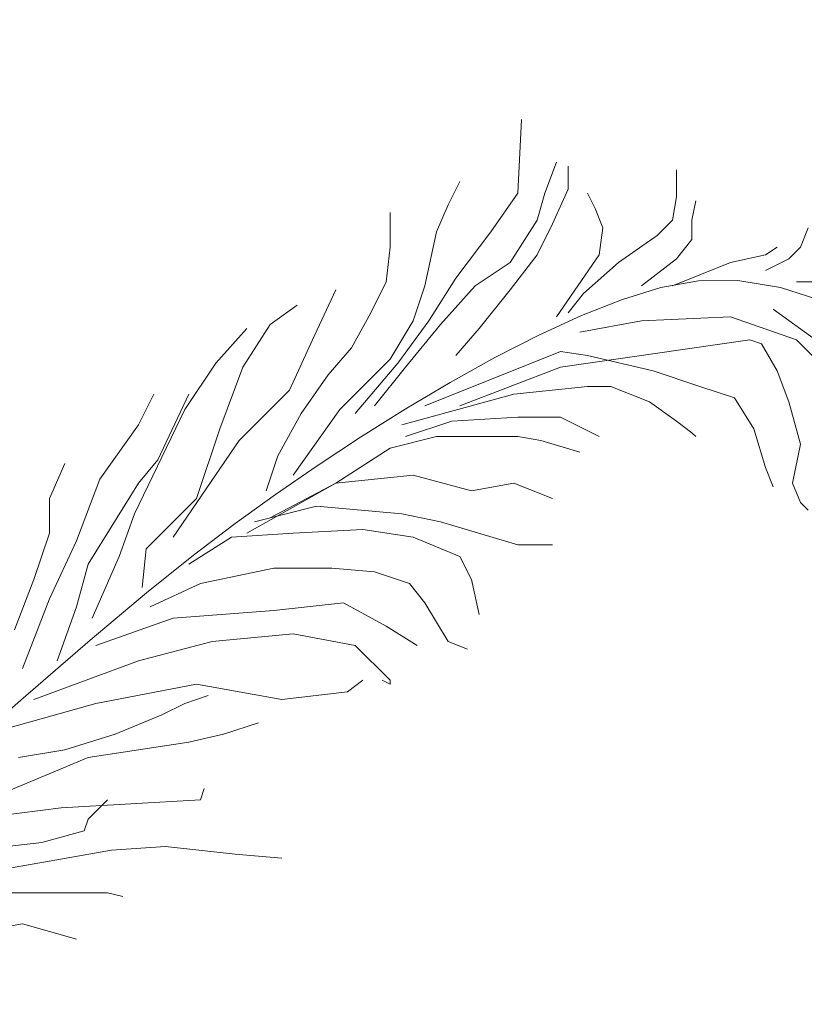
# Model space of a CAD drawing. Units: millimetres. Extents: x 595116 to 630915, y 909473 to 920225.
# Tile 62 of 134: x 629604.389 to 629608.928, y 919295.882 to 919301.582. Entities that reach past the tile are written whole.
import ezdxf

# ---------------------------------------------------------------- set-up
doc = ezdxf.new("R2010")
doc.units = ezdxf.units.MM
doc.layers.add('Dimension', color=3, linetype='Continuous', lineweight=18)
doc.layers.add('L-PLNT', color=85, linetype='Continuous', lineweight=13)
doc.styles.get("Standard").update_dxf_attribs({"font": 'arial.ttf'})
doc.dimstyles.new('ISO-25', dxfattribs={"dimtxt": 9, "dimasz": 6, "dimexe": 1.25, "dimexo": 0.625, "dimtad": 1, "dimlunit": 4, "dimtxsty": 'Standard', "dimcen": 2.5, "dimadec": 0, "dimazin": 0, "dimtfac": 1, "dimtmove": 0, "dimatfit": 3, "dimfxl": 1, "dimarcsym": 0})

# ---------------------------------------------------------------- blocks, each defined once
blk = doc.blocks.new('A$C4FB75ABC')
for p, q in [((4.1608, 3.5609), (4.1668, 3.6742)), ((4.2026, 3.5609), (4.2205, 3.6086)), ((4.2384, 3.5668), (4.2384, 3.6026)), ((4.4054, 3.5549), (4.4054, 3.5967)), ((4.0535, 3.543), (4.0714, 3.5788)), ((4.1191, 3.5013), (4.1608, 3.5609)), ((4.1907, 3.5192), (4.2026, 3.5609)), ((4.2145, 3.5132), (4.2384, 3.5668)), ((4.2801, 3.537), (4.2682, 3.5609)), ((4.3994, 3.5192), (4.4054, 3.5549)), ((4.0356, 3.5013), (4.0535, 3.543)), ((4.4293, 3.5192), (4.4352, 3.549)), ((3.964, 3.4774), (3.964, 3.5311)), ((4.2921, 3.5072), (4.2801, 3.537)), ((4.1489, 3.4536), (4.1907, 3.5192)), ((4.1907, 3.4655), (4.2145, 3.5132)), ((4.3756, 3.4953), (4.3994, 3.5192)), ((4.4293, 3.4893), (4.4293, 3.5192)), ((4.0177, 3.4178), (4.0356, 3.5013)), ((4.0654, 3.4297), (4.1191, 3.5013)), ((4.2861, 3.4655), (4.2921, 3.5072)), ((4.3159, 3.4536), (4.3756, 3.4953)), ((4.5963, 3.4774), (4.6082, 3.5072)), ((3.958, 3.4238), (3.964, 3.4774)), ((4.4054, 3.4595), (4.4293, 3.4893)), ((4.5426, 3.4655), (4.5605, 3.4774)), ((4.5784, 3.4595), (4.5963, 3.4774)), ((4.1489, 3.4118), (4.1907, 3.4655)), ((4.2205, 3.3701), (4.2861, 3.4655)), ((4.4889, 3.4536), (4.5426, 3.4655)), ((4.0952, 3.4178), (4.1489, 3.4536)), ((4.2622, 3.4059), (4.3159, 3.4536)), ((4.3517, 3.4178), (4.4054, 3.4595)), ((4.3994, 3.4178), (4.4889, 3.4536)), ((4.5426, 3.4416), (4.5784, 3.4595)), ((3.9342, 3.3761), (3.958, 3.4238)), ((3.9998, 3.3641), (4.0177, 3.4178)), ((4.0237, 3.3641), (4.0654, 3.4297)), ((4.0415, 3.3582), (4.0952, 3.4178)), ((4.3813, 3.4152), (4.4396, 3.4254)), ((4.4396, 3.4254), (4.5001, 3.426)), ((4.5001, 3.426), (4.5657, 3.4153)), ((4.5903, 3.4238), (4.6201, 3.4238)), ((3.8447, 3.3343), (3.8805, 3.4118)), ((4.1012, 3.3522), (4.1489, 3.4118)), ((4.2384, 3.3761), (4.2622, 3.4059)), ((4.322, 3.3969), (4.3813, 3.4152)), ((4.5657, 3.4153), (4.6395, 3.3917)), ((3.7791, 3.3582), (3.8208, 3.388)), ((4.2593, 3.3722), (4.322, 3.3969)), ((3.9044, 3.3224), (3.9342, 3.3761)), ((4.1935, 3.342), (4.2593, 3.3722)), ((4.5545, 3.382), (4.6858, 3.2866)), ((3.7373, 3.2926), (3.7791, 3.3582)), ((3.964, 3.3045), (3.9998, 3.3641)), ((3.9759, 3.2986), (4.0237, 3.3641)), ((3.9879, 3.2926), (4.0415, 3.3582)), ((4.2563, 3.3463), (4.3517, 3.3641)), ((4.3517, 3.3641), (4.4889, 3.3701)), ((4.4889, 3.3701), (4.5903, 3.3343)), ((3.6956, 3.2986), (3.7433, 3.3522)), ((4.0654, 3.3105), (4.1012, 3.3522)), ((4.1256, 3.3072), (4.1935, 3.342)), ((3.8089, 3.2568), (3.8447, 3.3343)), ((4.2265, 3.2926), (4.5187, 3.3343)), ((4.5187, 3.3343), (4.5366, 3.3284)), ((4.5366, 3.3284), (4.5605, 3.2866)), ((4.5903, 3.3343), (4.644, 3.2807)), ((3.8686, 3.2807), (3.9044, 3.3224)), ((4.0177, 3.233), (4.2265, 3.3164)), ((4.2265, 3.3164), (4.2682, 3.3105)), ((4.2682, 3.3105), (4.3696, 3.2866)), ((3.6479, 3.227), (3.6956, 3.2986)), ((3.8865, 3.227), (3.964, 3.3045)), ((3.9103, 3.2211), (3.9759, 3.2986)), ((4.0565, 3.2687), (4.1256, 3.3072)), ((3.7015, 3.1972), (3.7373, 3.2926)), ((3.8268, 3.2211), (3.8686, 3.2807)), ((3.9401, 3.233), (3.9879, 3.2926)), ((4.0714, 3.233), (4.2265, 3.2926)), ((4.3696, 3.2866), (4.4412, 3.2628)), ((4.5605, 3.2866), (4.5784, 3.2389)), ((3.9871, 3.2274), (4.0565, 3.2687)), ((3.5763, 3.2032), (3.6001, 3.2509)), ((3.6061, 3.1495), (3.6538, 3.2509)), ((3.7314, 3.1793), (3.8089, 3.2568)), ((3.9819, 3.2032), (4.1549, 3.2509)), ((4.1549, 3.2509), (4.2682, 3.2628)), ((4.2682, 3.2628), (4.304, 3.2628)), ((4.304, 3.2628), (4.3637, 3.2389)), ((4.4412, 3.2628), (4.4949, 3.2449)), ((4.3637, 3.2389), (4.4054, 3.2091)), ((4.4949, 3.2449), (4.5247, 3.1972)), ((4.5784, 3.2389), (4.5963, 3.1734)), ((3.5703, 3.066), (3.6479, 3.227)), ((3.791, 3.1555), (3.8268, 3.2211)), ((3.8149, 3.1257), (3.8865, 3.227)), ((3.9185, 3.1843), (3.9871, 3.2274)), ((3.9879, 3.1853), (4.0594, 3.2091)), ((4.0594, 3.2091), (4.1608, 3.2151)), ((4.1608, 3.2151), (4.2265, 3.2151)), ((4.2265, 3.2151), (4.2861, 3.1853)), ((4.4054, 3.2091), (4.4293, 3.1912)), ((3.5166, 3.1197), (3.5763, 3.2032)), ((3.6658, 3.0899), (3.7015, 3.1972)), ((4.4293, 3.1912), (4.4352, 3.1853)), ((4.5247, 3.1972), (4.5426, 3.1376)), ((3.63, 3.0303), (3.7314, 3.1793)), ((3.8516, 3.1401), (3.9185, 3.1843)), ((3.964, 3.1674), (4.0356, 3.1853)), ((4.0356, 3.1853), (4.1072, 3.1853)), ((4.1072, 3.1853), (4.1608, 3.1853)), ((4.1608, 3.1853), (4.1966, 3.1793)), ((4.1966, 3.1793), (4.2563, 3.1614)), ((3.8805, 3.1137), (3.964, 3.1674)), ((4.5963, 3.1734), (4.5844, 3.1137)), ((3.4391, 3.0899), (3.4629, 3.1436)), ((3.5763, 3.1137), (3.6061, 3.1495)), ((3.7731, 3.1018), (3.791, 3.1555)), ((3.7873, 3.0958), (3.8516, 3.1401)), ((4.5426, 3.1376), (4.5545, 3.1078)), ((3.4808, 3.0243), (3.5166, 3.1197)), ((3.4987, 2.9885), (3.5763, 3.1137)), ((3.7433, 3.0362), (3.8805, 3.1137)), ((3.7791, 3.0601), (3.8805, 3.1137)), ((3.8805, 3.1137), (3.9998, 3.1257)), ((3.9998, 3.1257), (4.0893, 3.1018)), ((4.0893, 3.1018), (4.1549, 3.1137)), ((4.1549, 3.1137), (4.2145, 3.0899)), ((4.5844, 3.1137), (4.5963, 3.0839)), ((3.4391, 3.0362), (3.4391, 3.0899)), ((3.5882, 3.0124), (3.6658, 3.0899)), ((3.7254, 3.0513), (3.7873, 3.0958)), ((4.5963, 3.0839), (4.6082, 3.072)), ((3.7552, 3.0541), (3.8507, 3.078)), ((3.8507, 3.078), (3.9819, 3.066)), ((3.5465, 3.0005), (3.5703, 3.066)), ((3.9819, 3.066), (4.0415, 3.0541)), ((4.0415, 3.0541), (4.1608, 3.0184)), ((3.6611, 3.0024), (3.7254, 3.0513)), ((3.8149, 3.0362), (3.9222, 3.0422)), ((3.9222, 3.0422), (3.9998, 3.0303)), ((3.4152, 2.9647), (3.4391, 3.0362)), ((3.4391, 2.9349), (3.4808, 3.0243)), ((3.6538, 2.9885), (3.7194, 3.0303)), ((3.7194, 3.0303), (3.8149, 3.0362)), ((3.9998, 3.0303), (4.0714, 3.0005)), ((3.5822, 2.9528), (3.5882, 3.0124)), ((4.1608, 3.0184), (4.2145, 3.0184)), ((3.5047, 2.9051), (3.5465, 3.0005)), ((3.5886, 2.9442), (3.6611, 3.0024)), ((4.0714, 3.0005), (4.0893, 2.9647)), ((3.4808, 2.923), (3.4987, 2.9885)), ((3.6717, 2.9587), (3.7851, 2.9826)), ((3.7851, 2.9826), (3.8745, 2.9826)), ((3.8745, 2.9826), (3.9401, 2.9766)), ((3.9401, 2.9766), (3.9938, 2.9587)), ((3.3854, 2.8872), (3.4152, 2.9647)), ((4.0893, 2.9647), (4.1012, 2.911)), ((3.5942, 2.923), (3.6717, 2.9587)), ((3.9938, 2.9587), (4.0177, 2.9289)), ((3.3973, 2.8276), (3.4391, 2.9349)), ((3.5019, 2.8714), (3.5886, 2.9442)), ((3.451, 2.8395), (3.4808, 2.923)), ((3.63, 2.9051), (3.7851, 2.917)), ((3.7851, 2.917), (3.8924, 2.9289)), ((3.8924, 2.9289), (3.958, 2.8932)), ((4.0177, 2.9289), (4.0535, 2.8693)), ((3.5107, 2.8633), (3.63, 2.9051)), ((3.958, 2.8932), (4.0058, 2.8633)), ((3.3951, 2.779), (3.5019, 2.8714)), ((3.6896, 2.8693), (3.8149, 2.8812)), ((3.8149, 2.8812), (3.9103, 2.8633)), ((3.5763, 2.8395), (3.6896, 2.8693)), ((3.9103, 2.8633), (3.964, 2.8097)), ((4.0535, 2.8693), (4.0833, 2.8574)), ((3.4152, 2.7799), (3.5763, 2.8395)), ((3.8984, 2.7918), (3.9222, 2.8097)), ((3.964, 2.8037), (3.9521, 2.8097)), ((3.964, 2.8097), (3.964, 2.8037)), ((3.5107, 2.7739), (3.6658, 2.8037)), ((3.6658, 2.8037), (3.797, 2.7799)), ((3.2623, 2.6619), (3.3951, 2.779)), ((3.6479, 2.7739), (3.6837, 2.7858)), ((3.797, 2.7799), (3.8984, 2.7918)), ((3.3615, 2.7322), (3.5107, 2.7739)), ((3.6121, 2.756), (3.6479, 2.7739)), ((3.5405, 2.7262), (3.6121, 2.756)), ((3.7075, 2.7262), (3.7612, 2.7441)), ((3.4629, 2.7024), (3.5405, 2.7262)), ((3.6538, 2.7143), (3.7075, 2.7262)), ((3.4987, 2.6904), (3.6538, 2.7143)), ((3.2422, 2.5831), (3.4987, 2.6904)), ((3.3914, 2.6904), (3.4629, 2.7024)), ((3.6717, 2.6249), (3.6777, 2.6428)), ((3.3198, 2.5951), (3.457, 2.6129)), ((3.457, 2.6129), (3.6717, 2.6249)), ((3.4987, 2.5951), (3.5286, 2.6249)), ((3.4928, 2.5772), (3.4987, 2.5951)), ((3.4272, 2.5593), (3.4928, 2.5772)), ((3.3198, 2.5474), (3.4272, 2.5593)), ((3.5345, 2.5474), (3.618, 2.5533)), ((3.618, 2.5533), (3.7254, 2.5414)), ((3.1289, 2.4758), (3.5345, 2.5474)), ((3.7254, 2.5414), (3.797, 2.5354)), ((3.3019, 2.4818), (3.4152, 2.4818)), ((3.4152, 2.4818), (3.5286, 2.4818)), ((3.5286, 2.4818), (3.5524, 2.4758)), ((3.3019, 2.4162), (3.3973, 2.4341)), ((3.3973, 2.4341), (3.4808, 2.4102))]:
    blk.add_line(p, q)
blk = doc.blocks.new('*D210')
at = {"layer": 'Defpoints', "color": 0, "transparency": 16777216}
for p in [(629586.2273, 919310.1229), (629593.9463, 919310.1229), (629586.2273, 919258.6624)]:
    blk.add_point(p, dxfattribs=at)
at = {"layer": 'Dimension', "color": 0, "lineweight": -2, "transparency": 16777216}
for p, q in [((629593.9463, 919310.1229), (629593.9463, 919449.6901)), ((629586.8523, 919310.1229), (629595.1963, 919310.1229)), ((629593.9463, 919264.6624), (629593.9463, 919304.1229)), ((629586.8523, 919258.6624), (629595.1963, 919258.6624))]:
    blk.add_line(p, q, dxfattribs=at)
at = {"layer": 'Dimension', "color": 0, "transparency": 16777216}
for points in [[(629592.9463, 919304.1229), (629594.9463, 919304.1229), (629593.9463, 919310.1229)], [(629592.9463, 919264.6624), (629594.9463, 919264.6624), (629593.9463, 919258.6624)]]:
    blk.add_solid(points, dxfattribs=at)
at = {"layer": 'Dimension', "color": 0, "transparency": 16777216, "insert": (629588.6617, 919382.9065), "char_height": 9, "attachment_point": 5, "rotation": 90}
blk.add_mtext('CANOPY 4\'-3 1/2" TYP.', dxfattribs=at)
blk = doc.blocks.new('*D216')
at = {"layer": 'Defpoints', "color": 0, "transparency": 16777216}
for p in [(629743.5408, 919411.9276), (629505.0408, 919411.8279), (629743.5408, 918832.3776)]:
    blk.add_point(p, dxfattribs=at)
at = {"layer": 'Dimension', "color": 0, "lineweight": -2, "transparency": 16777216}
for p, q in [((629743.5408, 919411.3026), (629743.5408, 918831.1276)), ((629505.0408, 919411.2029), (629505.0408, 918831.1276)), ((629511.0408, 918832.3776), (629737.5408, 918832.3776))]:
    blk.add_line(p, q, dxfattribs=at)
at = {"layer": 'Dimension', "color": 0, "transparency": 16777216}
for points in [[(629511.0408, 918833.3776), (629511.0408, 918831.3776), (629505.0408, 918832.3776)], [(629737.5408, 918833.3776), (629737.5408, 918831.3776), (629743.5408, 918832.3776)]]:
    blk.add_solid(points, dxfattribs=at)
at = {"layer": 'Dimension', "color": 0, "transparency": 16777216, "insert": (629624.2908, 918837.656), "char_height": 9, "attachment_point": 5}
blk.add_mtext('19\'-10 1/2"', dxfattribs=at)

msp = doc.modelspace()

# ---------------------------------------------------------------- block references
at = {"layer": 'L-PLNT', "xscale": 3.753413438031968, "yscale": 3.753413438031968, "zscale": 3.753413438031968}
msp.add_blockref('A$C4FB75ABC', (629591.6528, 919287.2124), dxfattribs=at)

# ---------------------------------------------------------------- dimensions: what is measured, and where the dimension line sits
at = {"layer": 'Dimension'}
dim = msp.add_linear_dim(base=(629593.9463, 919310.1229), p1=(629586.2273, 919258.6624), p2=(629586.2273, 919310.1229), angle=90, text='CANOPY <> TYP.', dimstyle='ISO-25', override={"dimdec": 1, "dimlfac": 1, "dimrnd": 0, "dimzin": 1, "dimdsep": 46, "dimlunit": 4, "dimfrac": 2}, dxfattribs=at)
dim.commit()
dim.dimension.update_dxf_attribs({"geometry": '*D210', "text_midpoint": (629588.6617, 919382.9065)})
dim = msp.add_linear_dim(base=(629743.5408, 918832.3776), p1=(629505.0408, 919411.8279), p2=(629743.5408, 919411.9276), dimstyle='ISO-25', override={"dimdec": 1, "dimlfac": 1, "dimrnd": 0, "dimzin": 1, "dimdsep": 46, "dimlunit": 4, "dimfrac": 2}, dxfattribs=at)
dim.commit()
dim.dimension.update_dxf_attribs({"geometry": '*D216', "text_midpoint": (629624.2908, 918837.656)})

doc.saveas('drawing.dxf')
